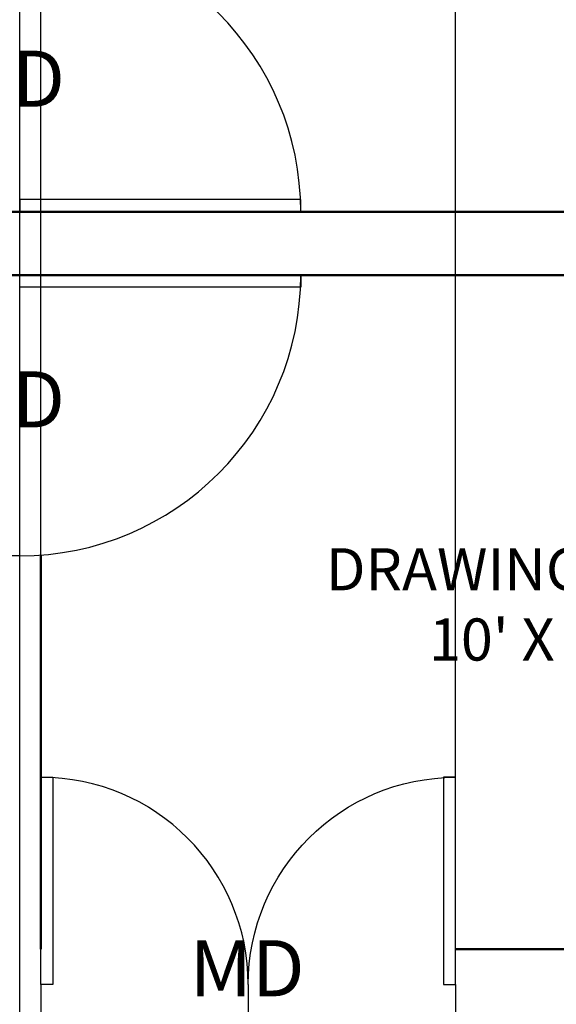
# Model space of a CAD drawing. Units: inches. Extents: x 37 to 824, y -700 to 234.
# Tile 39 of 77: x 296 to 372, y -215 to -75. Entities that reach past the tile are written whole.
import ezdxf

# ---------------------------------------------------------------- set-up
doc = ezdxf.new("R2010")
doc.units = ezdxf.units.IN
doc.header["$MEASUREMENT"] = 0
for name, color, linetype, lineweight in [('A-ANNO-DIMS', 2, 'Continuous', 18), ('A-ANNO-TEXT', 7, 'Continuous', 18), ('A-AREA-IDEN', 3, 'Continuous', 18), ('A-DOOR', 4, 'Continuous', 25), ('A-WALL', 2, 'Continuous', 50)]:
    doc.layers.add(name, color=color, linetype=linetype, lineweight=lineweight)
doc.styles.get("Standard").update_dxf_attribs({"font": 'arial.ttf'})
doc.dimstyles.get("Standard").update_dxf_attribs({"dimtxt": 0.18, "dimasz": 0.18, "dimexe": 0.18, "dimexo": 0.0625, "dimgap": 0.09, "dimtad": 0, "dimtih": 1, "dimtoh": 1, "dimdec": 1, "dimzin": 0, "dimdsep": 46, "dimlunit": 4, "dimtxsty": 'Standard', "dimcen": 0.09, "dimadec": 0, "dimazin": 0, "dimtfac": 1, "dimtdec": 1, "dimtofl": 0, "dimtmove": 0, "dimatfit": 3, "dimfxl": 1, "dimtolj": 1, "dimtzin": 0, "dimarcsym": 0})

# ---------------------------------------------------------------- blocks, each defined once
blk = doc.blocks.new('*U5')
for p, q in [((0, 0), (0, 6)), ((40, 0), (40, 6))]:
    blk.add_line(p, q)
blk.add_lwpolyline([(0, 0), (0, -40), (1.75, -40), (1.75, 0)], close=True)
blk.add_arc((0, 0), 40, 270, 0)
blk = doc.blocks.new('*U4')
for p, q in [((0, 0), (0, -100)), ((750, 0), (750, -100))]:
    blk.add_line(p, q)
blk.add_lwpolyline([(0, 0), (0, 750), (43.75, 750), (43.75, 0)], close=True)
blk.add_arc((0, 0), 750, 0, 90)
blk = doc.blocks.new('*U2')
for p, q in [((-40, 0), (-40, 6)), ((0, 0), (0, 6))]:
    blk.add_line(p, q)
blk.add_lwpolyline([(0, 0), (0, -40), (-1.75, -40), (-1.75, 0)], close=True)
blk.add_arc((0, 0), 40, 180, 270)
blk = doc.blocks.new('*D79')
at = {"layer": 'A-ANNO-DIMS', "color": 0, "lineweight": -2, "ltscale": 0.5, "transparency": 16777216}
for p, q in [((299.14, -62.02), (513.77, -62.02)), ((513.59, -62.2), (513.59, -81.78)), ((513.59, -101.73), (513.59, -82.15)), ((296.14, -101.91), (513.77, -101.91))]:
    blk.add_line(p, q, dxfattribs=at)
at = {"layer": 'A-ANNO-DIMS', "color": 0, "ltscale": 0.5, "transparency": 16777216}
for points in [[(513.56, -62.2), (513.62, -62.2), (513.59, -62.02)], [(513.56, -101.73), (513.62, -101.73), (513.59, -101.91)]]:
    blk.add_solid(points, dxfattribs=at)
at = {"layer": 'Defpoints', "color": 0, "ltscale": 0.5, "transparency": 16777216}
for p in [(299.08, -62.02), (296.08, -101.91), (513.59, -101.91)]:
    blk.add_point(p, dxfattribs=at)
at = {"layer": 'A-ANNO-DIMS', "color": 0, "ltscale": 0.5, "transparency": 16777216, "insert": (513.59, -81.97), "char_height": 0.18, "attachment_point": 5}
blk.add_mtext('\\A1;3\'-4"', dxfattribs=at)
blk = doc.blocks.new('*D82')
at = {"layer": 'A-ANNO-DIMS', "color": 0, "lineweight": -2, "ltscale": 0.5, "transparency": 16777216}
for p, q in [((299.08, -206.85), (299.08, 234.17)), ((299.26, 233.99), (328.2, 233.99)), ((357.95, 233.99), (329.01, 233.99)), ((358.13, -206.85), (358.13, 234.17))]:
    blk.add_line(p, q, dxfattribs=at)
at = {"layer": 'A-ANNO-DIMS', "color": 0, "ltscale": 0.5, "transparency": 16777216}
for points in [[(299.26, 234.02), (299.26, 233.96), (299.08, 233.99)], [(357.95, 234.02), (357.95, 233.96), (358.13, 233.99)]]:
    blk.add_solid(points, dxfattribs=at)
at = {"layer": 'Defpoints', "color": 0, "ltscale": 0.5, "transparency": 16777216}
for p in [(358.13, 233.99), (299.08, -206.91), (358.13, -206.91)]:
    blk.add_point(p, dxfattribs=at)
at = {"layer": 'A-ANNO-DIMS', "color": 0, "ltscale": 0.5, "transparency": 16777216, "insert": (328.6, 233.99), "char_height": 0.18, "attachment_point": 5}
blk.add_mtext('\\A1;4\'-11"', dxfattribs=at)
blk = doc.blocks.new('*D83')
at = {"layer": 'A-ANNO-DIMS', "color": 0, "lineweight": -2, "ltscale": 0.5, "transparency": 16777216}
for p, q in [((358.13, -206.85), (358.13, 234.17)), ((358.31, 233.99), (388.28, 233.99)), ((418.9, 233.99), (388.93, 233.99)), ((419.08, -206.85), (419.08, 234.17))]:
    blk.add_line(p, q, dxfattribs=at)
at = {"layer": 'A-ANNO-DIMS', "color": 0, "ltscale": 0.5, "transparency": 16777216}
for points in [[(358.31, 234.02), (358.31, 233.96), (358.13, 233.99)], [(418.9, 234.02), (418.9, 233.96), (419.08, 233.99)]]:
    blk.add_solid(points, dxfattribs=at)
at = {"layer": 'Defpoints', "color": 0, "ltscale": 0.5, "transparency": 16777216}
for p in [(419.08, 233.99), (358.13, -206.91), (419.08, -206.91)]:
    blk.add_point(p, dxfattribs=at)
at = {"layer": 'A-ANNO-DIMS', "color": 0, "ltscale": 0.5, "transparency": 16777216, "insert": (388.6, 233.99), "char_height": 0.18, "attachment_point": 5}
blk.add_mtext('\\A1;5\'-1"', dxfattribs=at)
blk = doc.blocks.new('*D87')
at = {"layer": 'A-ANNO-DIMS', "color": 0, "lineweight": -2, "ltscale": 0.5, "transparency": 16777216}
for p, q in [((216.08, -356.85), (216.08, 234.17)), ((216.26, 233.99), (255.75, 233.99)), ((295.9, 233.99), (256.41, 233.99)), ((296.08, -356.85), (296.08, 234.17))]:
    blk.add_line(p, q, dxfattribs=at)
at = {"layer": 'A-ANNO-DIMS', "color": 0, "ltscale": 0.5, "transparency": 16777216}
for points in [[(216.26, 234.02), (216.26, 233.96), (216.08, 233.99)], [(295.9, 234.02), (295.9, 233.96), (296.08, 233.99)]]:
    blk.add_solid(points, dxfattribs=at)
at = {"layer": 'Defpoints', "color": 0, "ltscale": 0.5, "transparency": 16777216}
for p in [(296.08, 233.99), (216.08, -356.91), (296.08, -356.91)]:
    blk.add_point(p, dxfattribs=at)
at = {"layer": 'A-ANNO-DIMS', "color": 0, "ltscale": 0.5, "transparency": 16777216, "insert": (256.08, 233.99), "char_height": 0.18, "attachment_point": 5}
blk.add_mtext('\\A1;6\'-8"', dxfattribs=at)

msp = doc.modelspace()

# ---------------------------------------------------------------- linework, layer by layer
at = {"layer": 'A-WALL'}
for p, q in [((419.08, -101.91), (290.08, -101.91)), ((419.08, -110.91), (290.08, -110.91)), ((299.08, -206.91), (299.08, -150.8)), ((419.08, -206.91), (358.13, -206.91))]:
    msp.add_line(p, q, dxfattribs=at)

# ---------------------------------------------------------------- block references
at = {"layer": 'A-DOOR', "rotation": 90}
for name, p in [('*U5', (296.08, -101.91)), ('*U2', (296.08, -110.91))]:
    msp.add_blockref(name, p, dxfattribs=at)
at = {"layer": 'A-DOOR', "yscale": 0.0393700787401575, "zscale": 0.0393700787401575}
for p, xscale in [((299.08, -211.97), 0.0393700787401575), ((358.13, -211.97), -0.0393700787401575)]:
    msp.add_blockref('*U4', p, dxfattribs=dict(at, xscale=xscale))

# ---------------------------------------------------------------- texts
at = {"layer": 'A-ANNO-TEXT'}
for s, p in [('D', (295.02, -86.95)), ('D', (295.02, -132.62)), ('MD', (320.27, -213.64))]:
    msp.add_text(s, height=8, dxfattribs=at).set_placement(p)
at = {"layer": 'A-AREA-IDEN', "insert": (339.67, -149.82), "char_height": 6, "attachment_point": 1}
msp.add_mtext_dynamic_manual_height_columns("DRAWING ROOM\\P        10' X 8'", width=88.3217, gutter_width=1, heights=[0], dxfattribs=at)

# ---------------------------------------------------------------- dimensions: what is measured, and where the dimension line sits
at = {"layer": 'A-ANNO-DIMS', "ltscale": 0.5}
for base, p1, p2, picture, middle in [((296.08, 233.99), (216.08, -356.91), (296.08, -356.91), '*D87', (256.08, 233.99)), ((358.1323, 233.9904), (299.0772, -206.9096), (358.1323, -206.9096), '*D82', (328.6047, 233.9904)), ((419.0772, 233.9904), (358.1323, -206.9096), (419.0772, -206.9096), '*D83', (388.6047, 233.9904))]:
    dim = msp.add_linear_dim(base=base, p1=p1, p2=p2, dimstyle='Standard', override={"dimdec": 1, "dimlfac": 1, "dimrnd": 0, "dimzin": 1, "dimdsep": 46, "dimlunit": 4, "dimfrac": 2}, dxfattribs=at)
    dim.commit()
    dim.dimension.update_dxf_attribs({"geometry": picture, "text_midpoint": middle})
dim = msp.add_linear_dim(base=(513.59, -101.91), p1=(299.08, -62.02), p2=(296.08, -101.91), angle=90, dimstyle='Standard', override={"dimdec": 1, "dimlfac": 1, "dimrnd": 0, "dimzin": 1, "dimdsep": 46, "dimlunit": 4, "dimfrac": 2}, dxfattribs=at)
dim.commit()
dim.dimension.update_dxf_attribs({"geometry": '*D79', "text_midpoint": (513.59, -81.97)})

doc.saveas('drawing.dxf')
